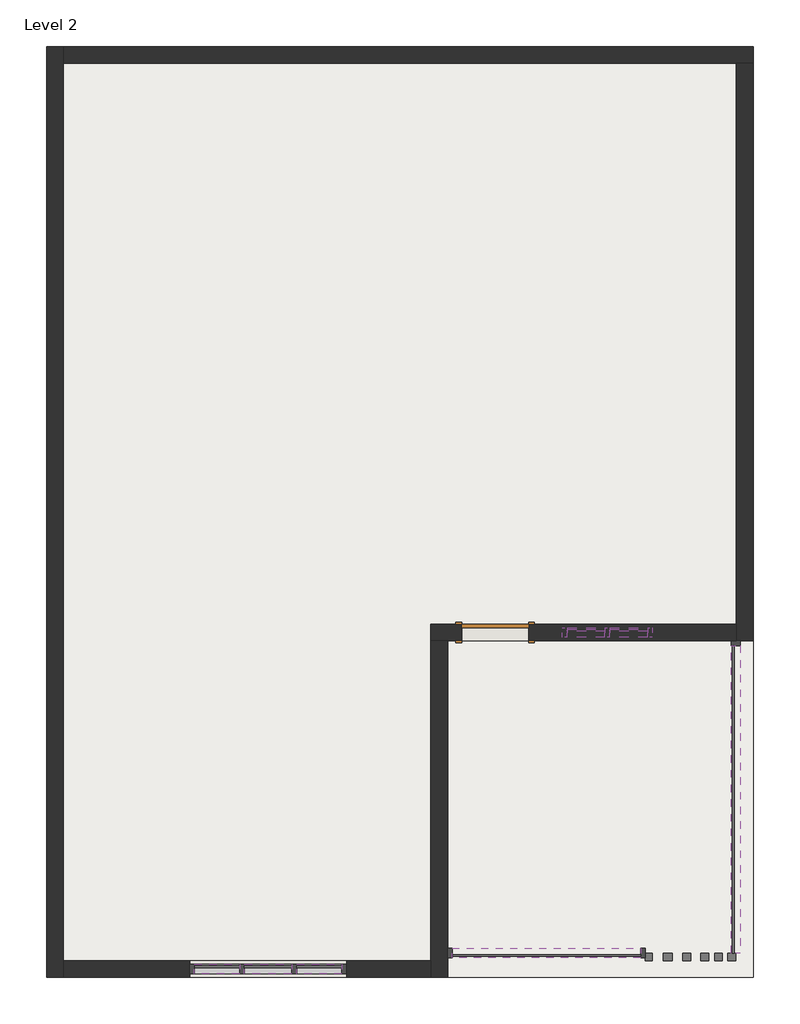
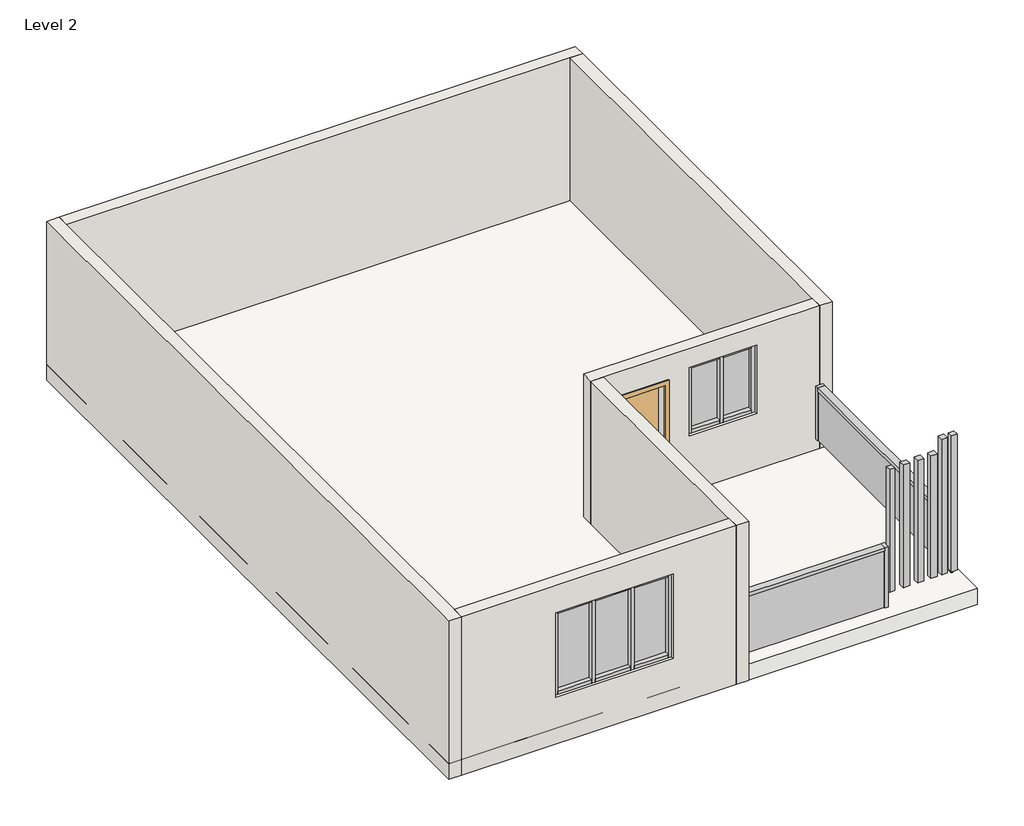
# One storey: 22 members, 7 plates, 6 walls, 1 door, 1 proxy, 1 roof.
"""IFC4 building model written with IfcOpenShell, lengths in millimetres."""

from ifc_helpers import new_model, si_unit, frame, origin, place, context, project, spatial, polyline, outline, extrude, faceted_brep, transform, mapped, element, save
from components import generic_models_2_generic_models_2_c977171b, door_0ca8825f, member_3f0e0172, member_5215b92c, member_0b7646a3, member_bef6d027, member_46459143, member_ae54c2fa, member_068505eb, member_ea8ac20a, member_6a413f91, member_86c371d5, member_0bcad3a7, system_panel_glazed_2c9823a4, system_panel_glazed_98683e45, system_panel_glazed_4a8c201a, system_panel_glazed_e2412059, system_panel_glazed_0c970258

model = new_model("IFC4")

# Units and contexts
model_context = context("Model", 3, world=origin())
ifc_project = project(units=[si_unit("LENGTHUNIT", "METRE", prefix="MILLI")], contexts=[model_context])

# Site, building, storey
site = spatial("IfcSite", under=ifc_project)
building = spatial("IfcBuilding", under=site)
storey = spatial("IfcBuildingStorey", under=building, Name="Level 2", Elevation=3048.0)

# Proxy
placement = place(None, origin())
generic_models_2_generic_models_2_shape = generic_models_2_generic_models_2_c977171b(model_context)
element("IfcBuildingElementProxy", 1, Name="Generic Models 2 : Generic Models 2", ObjectType="Generic Models 2 : Generic Models 2", at=placement, inside=storey, context=model_context, shape_type="MappedRepresentation", body=[
    mapped(generic_models_2_generic_models_2_shape, transform((0.0, 0.0, 0.0), x_axis=(1.0, 0.0, 0.0), y_axis=(0.0, 1.0, 0.0), z_axis=(0.0, 0.0, 1.0))),
])

# Door
door_shape = door_0ca8825f(model_context)
element("IfcDoor", 2, ObjectType="Single-Flush : 36\" x 84\"", at=placement, inside=storey, context=model_context, shape_type="MappedRepresentation", body=[
    mapped(door_shape, transform((-11082.387855, -7781.0768247, 3429.0), x_axis=(1.0, 0.0, 0.0), y_axis=(0.0, 1.0, 0.0), z_axis=(0.0, 0.0, 1.0))),
])

# Members
member_shape = member_3f0e0172(model_context)
element("IfcMember", 3, ObjectType="Rectangular Mullion : 2.5\" x 5\" rectangular", at=placement, inside=storey, context=model_context, shape_type="MappedRepresentation", body=[
    mapped(member_shape, transform((-13781.137855, -12353.0768247, 3946.5178454), x_axis=(0.0, 0.0, -1.0), y_axis=(0.0, -1.0, 0.0), z_axis=(-1.0, 0.0, 0.0))),
])
element("IfcMember", 4, ObjectType="Rectangular Mullion : 2.5\" x 5\" rectangular", at=placement, inside=storey, context=model_context, shape_type="MappedRepresentation", body=[
    mapped(member_shape, transform((-15171.787855, -12353.0768247, 3946.5178454), x_axis=(0.0, 0.0, -1.0), y_axis=(0.0, -1.0, 0.0), z_axis=(-1.0, 0.0, 0.0))),
])
member_2_shape = member_5215b92c(model_context)
element("IfcMember", 5, ObjectType="Rectangular Mullion : 2.5\" x 5\" rectangular", at=placement, inside=storey, context=model_context, shape_type="MappedRepresentation", body=[
    mapped(member_2_shape, transform((-14492.337855, -12353.0768247, 3946.5178454), x_axis=(0.0, 0.0, -1.0), y_axis=(0.0, -1.0, 0.0), z_axis=(-1.0, 0.0, 0.0))),
])
element("IfcMember", 6, ObjectType="Rectangular Mullion : 2.5\" x 5\" rectangular", at=placement, inside=storey, context=model_context, shape_type="MappedRepresentation", body=[
    mapped(member_2_shape, transform((-13844.637855, -12353.0768247, 5570.4532246), x_axis=(0.0, 0.0, 1.0), y_axis=(0.0, -1.0, 0.0), z_axis=(1.0, 0.0, 0.0))),
])
element("IfcMember", 7, ObjectType="Rectangular Mullion : 2.5\" x 5\" rectangular", at=placement, inside=storey, context=model_context, shape_type="MappedRepresentation", body=[
    mapped(member_shape, transform((-14555.837855, -12353.0768247, 5570.4532246), x_axis=(0.0, 0.0, 1.0), y_axis=(0.0, -1.0, 0.0), z_axis=(1.0, 0.0, 0.0))),
])
element("IfcMember", 8, ObjectType="Rectangular Mullion : 2.5\" x 5\" rectangular", at=placement, inside=storey, context=model_context, shape_type="MappedRepresentation", body=[
    mapped(member_shape, transform((-13165.187855, -12353.0768247, 5570.4532246), x_axis=(0.0, 0.0, 1.0), y_axis=(0.0, -1.0, 0.0), z_axis=(1.0, 0.0, 0.0))),
])
member_3_shape = member_0b7646a3(model_context)
element("IfcMember", 9, ObjectType="Rectangular Mullion : 2.5\" x 5\" rectangular", at=placement, inside=storey, context=model_context, shape_type="MappedRepresentation", body=[
    mapped(member_3_shape, transform((-9526.637855, -7781.0768247, 4423.8451348), x_axis=(0.0, 0.0, -1.0), y_axis=(0.0, -1.0, 0.0), z_axis=(-1.0, 0.0, 0.0))),
])
element("IfcMember", 10, ObjectType="Rectangular Mullion : 2.5\" x 5\" rectangular", at=placement, inside=storey, context=model_context, shape_type="MappedRepresentation", body=[
    mapped(member_3_shape, transform((-10104.487855, -7781.0768247, 4423.8451348), x_axis=(0.0, 0.0, -1.0), y_axis=(0.0, -1.0, 0.0), z_axis=(-1.0, 0.0, 0.0))),
])
element("IfcMember", 11, ObjectType="Rectangular Mullion : 2.5\" x 5\" rectangular", at=placement, inside=storey, context=model_context, shape_type="MappedRepresentation", body=[
    mapped(member_3_shape, transform((-9590.137855, -7781.0768247, 5735.8915212), x_axis=(0.0, 0.0, 1.0), y_axis=(0.0, -1.0, 0.0), z_axis=(1.0, 0.0, 0.0))),
])
element("IfcMember", 12, ObjectType="Rectangular Mullion : 2.5\" x 5\" rectangular", at=placement, inside=storey, context=model_context, shape_type="MappedRepresentation", body=[
    mapped(member_3_shape, transform((-9012.287855, -7781.0768247, 5735.8915212), x_axis=(0.0, 0.0, 1.0), y_axis=(0.0, -1.0, 0.0), z_axis=(1.0, 0.0, 0.0))),
])
member_4_shape = member_bef6d027(model_context)
element("IfcMember", 13, ObjectType="Rectangular Mullion : 2.5\" x 5\" rectangular", at=placement, inside=storey, context=model_context, shape_type="MappedRepresentation", body=[
    mapped(member_4_shape, transform((-14524.087855, -12353.0768247, 3946.5178454), x_axis=(1.0, 0.0, 0.0), y_axis=(0.0, -1.0, 0.0), z_axis=(0.0, 0.0, -1.0))),
])
element("IfcMember", 14, ObjectType="Rectangular Mullion : 2.5\" x 5\" rectangular", at=placement, inside=storey, context=model_context, shape_type="MappedRepresentation", body=[
    mapped(member_4_shape, transform((-13812.887855, -12353.0768247, 3946.5178454), x_axis=(1.0, 0.0, 0.0), y_axis=(0.0, -1.0, 0.0), z_axis=(0.0, 0.0, -1.0))),
])
member_5_shape = member_46459143(model_context)
element("IfcMember", 15, ObjectType="Rectangular Mullion : 2.5\" x 5\" rectangular", at=placement, inside=storey, context=model_context, shape_type="MappedRepresentation", body=[
    mapped(member_5_shape, transform((-15235.287855, -12353.0768247, 5570.4532246), x_axis=(-1.0, 0.0, 0.0), y_axis=(0.0, -1.0, 0.0), z_axis=(0.0, 0.0, 1.0))),
])
element("IfcMember", 16, ObjectType="Rectangular Mullion : 2.5\" x 5\" rectangular", at=placement, inside=storey, context=model_context, shape_type="MappedRepresentation", body=[
    mapped(member_5_shape, transform((-13101.687855, -12353.0768247, 3946.5178454), x_axis=(1.0, 0.0, 0.0), y_axis=(0.0, -1.0, 0.0), z_axis=(0.0, 0.0, -1.0))),
])
member_6_shape = member_ae54c2fa(model_context)
element("IfcMember", 17, ObjectType="Rectangular Mullion : 2.5\" x 5\" rectangular", at=placement, inside=storey, context=model_context, shape_type="MappedRepresentation", body=[
    mapped(member_6_shape, transform((-9558.387855, -7781.0768247, 4423.8451348), x_axis=(1.0, 0.0, 0.0), y_axis=(0.0, -1.0, 0.0), z_axis=(0.0, 0.0, -1.0))),
])
member_7_shape = member_068505eb(model_context)
element("IfcMember", 18, ObjectType="Rectangular Mullion : 2.5\" x 5\" rectangular", at=placement, inside=storey, context=model_context, shape_type="MappedRepresentation", body=[
    mapped(member_7_shape, transform((-10167.987855, -7781.0768247, 5735.8915212), x_axis=(-1.0, 0.0, 0.0), y_axis=(0.0, -1.0, 0.0), z_axis=(0.0, 0.0, 1.0))),
])
element("IfcMember", 19, ObjectType="Rectangular Mullion : 2.5\" x 5\" rectangular", at=placement, inside=storey, context=model_context, shape_type="MappedRepresentation", body=[
    mapped(member_7_shape, transform((-8948.787855, -7781.0768247, 4423.8451348), x_axis=(1.0, 0.0, 0.0), y_axis=(0.0, -1.0, 0.0), z_axis=(0.0, 0.0, -1.0))),
])
member_8_shape = member_ea8ac20a(model_context)
element("IfcMember", 20, ObjectType="Rectangular Mullion : 2.5\" x 5\" rectangular", at=placement, inside=storey, context=model_context, shape_type="MappedRepresentation", body=[
    mapped(member_8_shape, transform((-11730.087855, -12137.1768247, 3048.0), x_axis=(-1.0, 0.0, 0.0), y_axis=(0.0, 1.0, 0.0), z_axis=(0.0, 0.0, -1.0))),
])
member_9_shape = member_6a413f91(model_context)
element("IfcMember", 21, ObjectType="Rectangular Mullion : 2.5\" x 5\" rectangular", at=placement, inside=storey, context=model_context, shape_type="MappedRepresentation", body=[
    mapped(member_9_shape, transform((-11666.587855, -12137.1768247, 4511.715679), x_axis=(0.0, 0.0, 1.0), y_axis=(0.0, 1.0, 0.0), z_axis=(-1.0, 0.0, 0.0))),
])
element("IfcMember", 22, ObjectType="Rectangular Mullion : 2.5\" x 5\" rectangular", at=placement, inside=storey, context=model_context, shape_type="MappedRepresentation", body=[
    mapped(member_8_shape, transform((-9042.1407178, -12137.1768247, 4511.715679), x_axis=(1.0, 0.0, 0.0), y_axis=(0.0, 1.0, 0.0), z_axis=(0.0, 0.0, 1.0))),
])
member_10_shape = member_86c371d5(model_context)
element("IfcMember", 23, ObjectType="Rectangular Mullion : 2.5\" x 5\" rectangular", at=placement, inside=storey, context=model_context, shape_type="MappedRepresentation", body=[
    mapped(member_10_shape, transform((-7813.9345733, -7958.8768247, 4578.0887128), x_axis=(0.0, 0.0, 1.0), y_axis=(1.0, 0.0, 0.0), z_axis=(0.0, 1.0, 0.0))),
])
member_11_shape = member_0bcad3a7(model_context)
element("IfcMember", 24, ObjectType="Rectangular Mullion : 2.5\" x 5\" rectangular", at=placement, inside=storey, context=model_context, shape_type="MappedRepresentation", body=[
    mapped(member_11_shape, transform((-7813.9345733, -7895.3768247, 3556.6620216), x_axis=(0.0, 1.0, 0.0), y_axis=(1.0, 0.0, 0.0), z_axis=(0.0, 0.0, -1.0))),
])

# Plates
system_panel_glazed_shape = system_panel_glazed_2c9823a4(model_context)
element("IfcPlate", 25, ObjectType="System Panel : Glazed", at=placement, inside=storey, context=model_context, shape_type="MappedRepresentation", body=[
    mapped(system_panel_glazed_shape, transform((-14863.812855, -12353.0768247, 4010.0178454), x_axis=(1.0, 0.0, 0.0), y_axis=(0.0, 1.0, 0.0), z_axis=(0.0, 0.0, 1.0))),
])
element("IfcPlate", 26, ObjectType="System Panel : Glazed", at=placement, inside=storey, context=model_context, shape_type="MappedRepresentation", body=[
    mapped(system_panel_glazed_shape, transform((-13473.162855, -12353.0768247, 4010.0178454), x_axis=(1.0, 0.0, 0.0), y_axis=(0.0, 1.0, 0.0), z_axis=(0.0, 0.0, 1.0))),
])
system_panel_glazed_2_shape = system_panel_glazed_98683e45(model_context)
element("IfcPlate", 27, ObjectType="System Panel : Glazed", at=placement, inside=storey, context=model_context, shape_type="MappedRepresentation", body=[
    mapped(system_panel_glazed_2_shape, transform((-14168.487855, -12353.0768247, 4010.0178454), x_axis=(1.0, 0.0, 0.0), y_axis=(0.0, 1.0, 0.0), z_axis=(0.0, 0.0, 1.0))),
])
system_panel_glazed_3_shape = system_panel_glazed_4a8c201a(model_context)
element("IfcPlate", 28, ObjectType="System Panel : Glazed", at=placement, inside=storey, context=model_context, shape_type="MappedRepresentation", body=[
    mapped(system_panel_glazed_3_shape, transform((-9847.312855, -7781.0768247, 4487.3451348), x_axis=(1.0, 0.0, 0.0), y_axis=(0.0, 1.0, 0.0), z_axis=(0.0, 0.0, 1.0))),
])
element("IfcPlate", 29, ObjectType="System Panel : Glazed", at=placement, inside=storey, context=model_context, shape_type="MappedRepresentation", body=[
    mapped(system_panel_glazed_3_shape, transform((-9269.462855, -7781.0768247, 4487.3451348), x_axis=(1.0, 0.0, 0.0), y_axis=(0.0, 1.0, 0.0), z_axis=(0.0, 0.0, 1.0))),
])
system_panel_glazed_4_shape = system_panel_glazed_e2412059(model_context)
element("IfcPlate", 30, ObjectType="System Panel : Glazed", at=placement, inside=storey, context=model_context, shape_type="MappedRepresentation", body=[
    mapped(system_panel_glazed_4_shape, transform((-10386.1142864, -12137.1768247, 3048.0), x_axis=(-1.0, 0.0, 0.0), y_axis=(0.0, -1.0, 0.0), z_axis=(0.0, 0.0, 1.0))),
])
system_panel_glazed_5_shape = system_panel_glazed_0c970258(model_context)
element("IfcPlate", 31, ObjectType="System Panel : Glazed", at=placement, inside=storey, context=model_context, shape_type="MappedRepresentation", body=[
    mapped(system_panel_glazed_5_shape, transform((-7813.9345733, -10048.0268247, 3556.6620216), x_axis=(0.0, 1.0, 0.0), y_axis=(-1.0, 0.0, 0.0), z_axis=(0.0, 0.0, 1.0))),
])

# Roof
element("IfcRoof", 32, ObjectType="Generic - 12\"", at=placement, inside=storey, context=model_context, shape_type="SweptSolid", body=[
    extrude(outline(polyline([(-17178.387855, 181.8231753), (-7577.187855, 181.8231753), (-7577.187855, -12467.3768247), (-17178.387855, -12467.3768247), (-17178.387855, 181.8231753)])), frame((0.0, 0.0, 3048.0), z_axis=(0.0, 0.0, 1.0), x_axis=(1.0, 0.0, 0.0)), (0.0, 0.0, 1.0), 304.8),
])

# Walls
element("IfcWall", 33, ObjectType="9\"", at=placement, inside=storey, context=model_context, shape_type="Brep", body=[
    faceted_brep([(-16949.787855, -12467.3768247, 3048.0), (-16949.787855, -12238.7768247, 3048.0), (-16949.787855, -46.7768247, 3048.0), (-16949.787855, 181.8231753, 3048.0), (-16949.787855, 181.8231753, 6096.0), (-16949.787855, -46.7768247, 6096.0), (-16949.787855, -12238.7768247, 6096.0), (-16949.787855, -12467.3768247, 6096.0), (-17178.387855, -12467.3768247, 3048.0), (-17178.387855, -12467.3768247, 6096.0), (-17178.387855, 181.8231753, 6096.0), (-17178.387855, 181.8231753, 3048.0)], [[[0, 1, 2, 3, 4, 5, 6, 7]], [[8, 9, 10, 11]], [[3, 2, 1, 0, 8, 11]], [[7, 6, 5, 4, 10, 9]], [[4, 3, 11, 10]], [[0, 7, 9, 8]]]),
])
element("IfcWall", 34, ObjectType="9\"", at=placement, inside=storey, context=model_context, shape_type="Brep", body=[
    faceted_brep([(-16949.787855, -46.7768247, 3048.0), (-7805.787855, -46.7768247, 3048.0), (-7577.187855, -46.7768247, 3048.0), (-7577.187855, -46.7768247, 6096.0), (-7805.787855, -46.7768247, 6096.0), (-16949.787855, -46.7768247, 6096.0), (-16949.787855, 181.8231753, 3048.0), (-16949.787855, 181.8231753, 6096.0), (-7577.187855, 181.8231753, 6096.0), (-7577.187855, 181.8231753, 3048.0)], [[[0, 1, 2, 3, 4, 5]], [[6, 7, 8, 9]], [[2, 1, 0, 6, 9]], [[5, 4, 3, 8, 7]], [[0, 5, 7, 6]], [[3, 2, 9, 8]]]),
])
element("IfcWall", 35, ObjectType="9\"", at=placement, inside=storey, context=model_context, shape_type="Brep", body=[
    faceted_brep([(-7805.787855, -46.7768247, 3048.0), (-7805.787855, -7666.7768247, 3048.0), (-7805.787855, -7895.3768247, 3048.0), (-7805.787855, -7895.3768247, 6096.0), (-7805.787855, -7666.7768247, 6096.0), (-7805.787855, -46.7768247, 6096.0), (-7577.187855, -46.7768247, 3048.0), (-7577.187855, -46.7768247, 6096.0), (-7577.187855, -7895.3768247, 6096.0), (-7577.187855, -7895.3768247, 3048.0)], [[[0, 1, 2, 3, 4, 5]], [[6, 7, 8, 9]], [[2, 1, 0, 6, 9]], [[5, 4, 3, 8, 7]], [[0, 5, 7, 6]], [[3, 2, 9, 8]]]),
])
element("IfcWall", 36, ObjectType="9\"", at=placement, inside=storey, context=model_context, shape_type="Brep", body=[
    faceted_brep([(-7805.787855, -7666.7768247, 3048.0), (-11958.687855, -7666.7768247, 3048.0), (-11958.687855, -7666.7768247, 6096.0), (-7805.787855, -7666.7768247, 6096.0), (-11539.587855, -7666.7768247, 3429.0), (-10625.187855, -7666.7768247, 3429.0), (-10625.187855, -7666.7768247, 5562.6), (-11539.587855, -7666.7768247, 5562.6), (-10167.987855, -7666.7768247, 5735.8915212), (-10167.987855, -7666.7768247, 4423.8451348), (-8948.787855, -7666.7768247, 4423.8451348), (-8948.787855, -7666.7768247, 5735.8915212), (-11958.687855, -7895.3768247, 3048.0), (-11730.087855, -7895.3768247, 3048.0), (-7805.787855, -7895.3768247, 3048.0), (-7805.787855, -7895.3768247, 6096.0), (-11730.087855, -7895.3768247, 6096.0), (-11958.687855, -7895.3768247, 6096.0), (-11539.587855, -7895.3768247, 3429.0), (-11539.587855, -7895.3768247, 5562.6), (-10625.187855, -7895.3768247, 5562.6), (-10625.187855, -7895.3768247, 3429.0), (-10167.987855, -7895.3768247, 4423.8451348), (-10167.987855, -7895.3768247, 5735.8915212), (-8948.787855, -7895.3768247, 5735.8915212), (-8948.787855, -7895.3768247, 4423.8451348)], [[[0, 1, 2, 3], [4, 5, 6, 7], [8, 9, 10, 11]], [[12, 13, 14, 15, 16, 17], [18, 19, 20, 21], [22, 23, 24, 25]], [[1, 0, 14, 13, 12]], [[3, 2, 17, 16, 15]], [[0, 3, 15, 14]], [[2, 1, 12, 17]], [[5, 4, 18, 21]], [[6, 5, 21, 20]], [[7, 6, 20, 19]], [[4, 7, 19, 18]], [[22, 9, 8, 23]], [[23, 8, 11, 24]], [[24, 11, 10, 25]], [[9, 22, 25, 10]]]),
])
element("IfcWall", 37, ObjectType="9\"", at=placement, inside=storey, context=model_context, shape_type="Brep", body=[
    faceted_brep([(-11958.687855, -7895.3768247, 3048.0), (-11958.687855, -12238.7768247, 3048.0), (-11958.687855, -12467.3768247, 3048.0), (-11958.687855, -12467.3768247, 6096.0), (-11958.687855, -12238.7768247, 6096.0), (-11958.687855, -7895.3768247, 6096.0), (-11730.087855, -7895.3768247, 3048.0), (-11730.087855, -7895.3768247, 6096.0), (-11730.087855, -12467.3768247, 6096.0), (-11730.087855, -12467.3768247, 3048.0)], [[[0, 1, 2, 3, 4, 5]], [[6, 7, 8, 9]], [[2, 1, 0, 6, 9]], [[5, 4, 3, 8, 7]], [[0, 5, 7, 6]], [[3, 2, 9, 8]]]),
])
element("IfcWall", 38, ObjectType="9\"", at=placement, inside=storey, context=model_context, shape_type="SweptSolid", body=[
    extrude(outline(polyline([(3048.0, -16949.787855), (3048.0, -11958.687855), (6096.0, -11958.687855), (6096.0, -16949.787855), (3048.0, -16949.787855)]), holes=[polyline([(3946.5178454, -15235.287855), (5570.4532246, -15235.287855), (5570.4532246, -13101.687855), (3946.5178454, -13101.687855), (3946.5178454, -15235.287855)])]), frame((0.0, -12467.3768247, 0.0), z_axis=(0.0, 1.0, 0.0), x_axis=(0.0, 0.0, 1.0)), (0.0, 0.0, 1.0), 228.6),
])

save(model, "model.ifc")

# Revit data of these elements
# Type "Single-Flush : 36\" x 84\""
#   Type Mark = "1"
#   Construction Type Id = "MDOOR"
#   Assembly Code = "C1020"
#   Analytic Construction = "Metal"
#   Thickness = 0' - 2"
#   Heat Transfer Coefficient (U) = 0.651978 BTU/(h·ft²·°F)
#   Height = 7' - 0"
#   Trim Projection Ext = 0' - 1"
#   Trim Projection Int = 0' - 1"
#   Trim Width = 0' - 3"
#   Width = 3' - 0"
#   Define Thermal Properties by = 1
#   Define Thermal Properties by = 1
#   Door Material = Door - Panel
#   Frame Material = Door - Frame
#   Visual Light Transmittance = 0
#   Solar Heat Gain Coefficient = 0
#   Function = (empty or 0)
#   Wall Closure = (empty or 0)
# Type "Rectangular Mullion : 2.5\" x 5\" rectangular"
#   built-in parameter 1007304 = 0.416667 (stored number, unit not read)
#   built-in parameter 1007301 = 0.104167 (stored number, unit not read)
#   built-in parameter 1007300 = 0.104167 (stored number, unit not read)
# Type "System Panel : Glazed"
#   Construction Type Id = "GSP4R"
#   Analytic Construction = "1/8 in Pilkington single glazing"
#   Visual Light Transmittance = 0.9
#   Solar Heat Gain Coefficient = 0.86
#   Heat Transfer Coefficient (U) = 1.18115 BTU/(h·ft²·°F)
#   Define Thermal Properties by = 1
# Type "Generic - 12\""
#   Assembly Code = "B1020"
#   Layers, outside or top first: 1' - 0" no material (function 1)
# Type "9\""
#   Assembly Code = "B2010"
#   Layers, outside or top first: 0' - 9" no material (function 1)
# Element 1 (IfcBuildingElementProxy, "Generic Models 2 : Generic Models 2")
#   Phase Created = New Construction
# Element 2 (IfcDoor, "Single-Flush : 36\" x 84\"")
#   Phase Created = New Construction
#   Materials on its faces: "Door - Frame", "Door - Panel"
# Elements 3, 4, 5, 6, 7, 8, 9, 10, 11, 12, 13, 14, 15, 16, 17, 18, 19, 20, 21, 22, 23, 24 (IfcMember, "Rectangular Mullion : 2.5\" x 5\" rectangular")
#   Phase Created = New Construction
#   Materials on its faces: "Aluminum"
# Elements 25, 26, 27, 28, 29, 30, 31 (IfcPlate, "System Panel : Glazed")
#   Phase Created = New Construction
#   Materials on its faces: "Glass"
# Element 32 (IfcRoof, "Generic - 12\"")
#   built-in parameter 1001705 = 11 (stored number, unit not read)
#   built-in parameter 1001710 = 33615
#   Phase Created = New Construction
#   Materials on its faces: "Default Roof"
# Elements 33, 34, 35, 36, 37, 38 (IfcWall, "9\"")
#   Top Offset = 0' - 0"
#   Base Offset = 0' - 0"
#   Unconnected Height = 10' - 0"
#   wall height = 10' - 0"
#   Phase Created = New Construction
#   Base Constraint = Level 2
#   Materials on its faces: "Default Wall"
# Materials
#   "Door - Panel": class "Wood", colour RGB 210 159 95, transparency 0, Cost = 0
#   "Door - Frame": colour RGB 118 70 51, transparency 0, Cost = 0
#   "Aluminum": class "Metal", colour RGB 247 247 247, transparency 0, Description = "Aluminum 6061", Cost = 0
#   "Glass": class "Glass", colour RGB 0 128 192, transparency 0.75, Description = "Soda Lime Glass", Cost = 0
#   "Default Roof": colour RGB 88 101 114, transparency 0, Cost = 0
#   "Default Wall": colour RGB 128 128 128, transparency 0, Cost = 0
